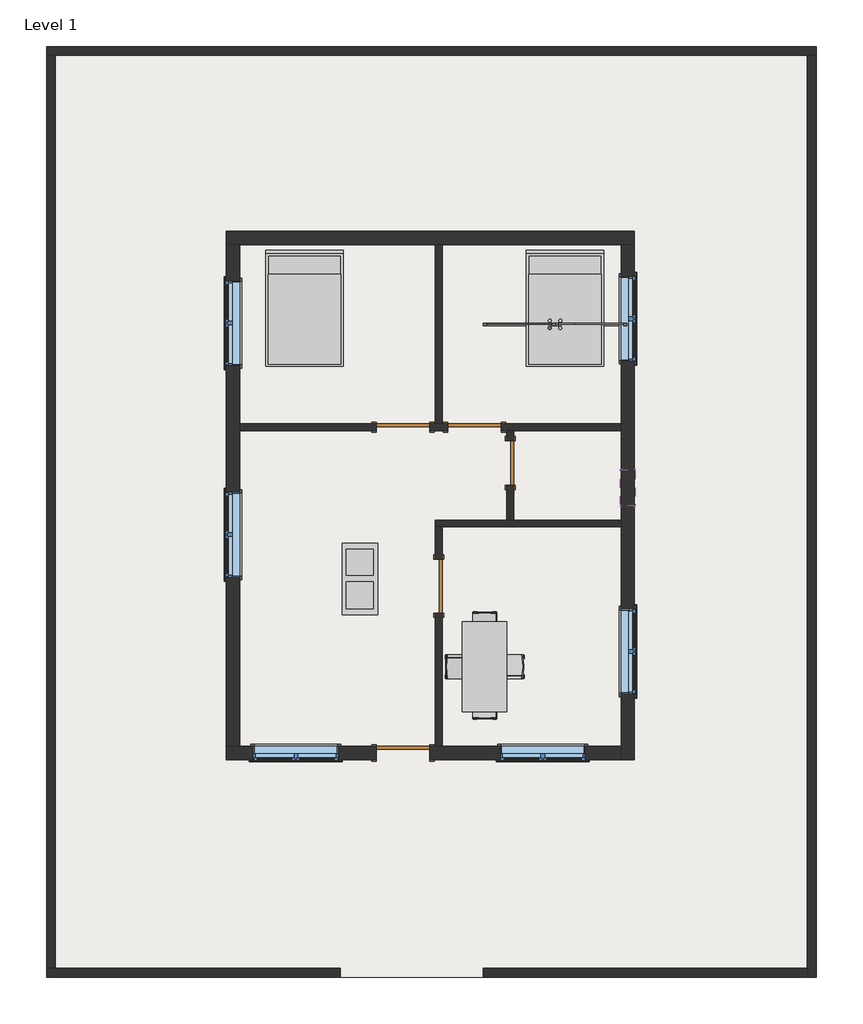
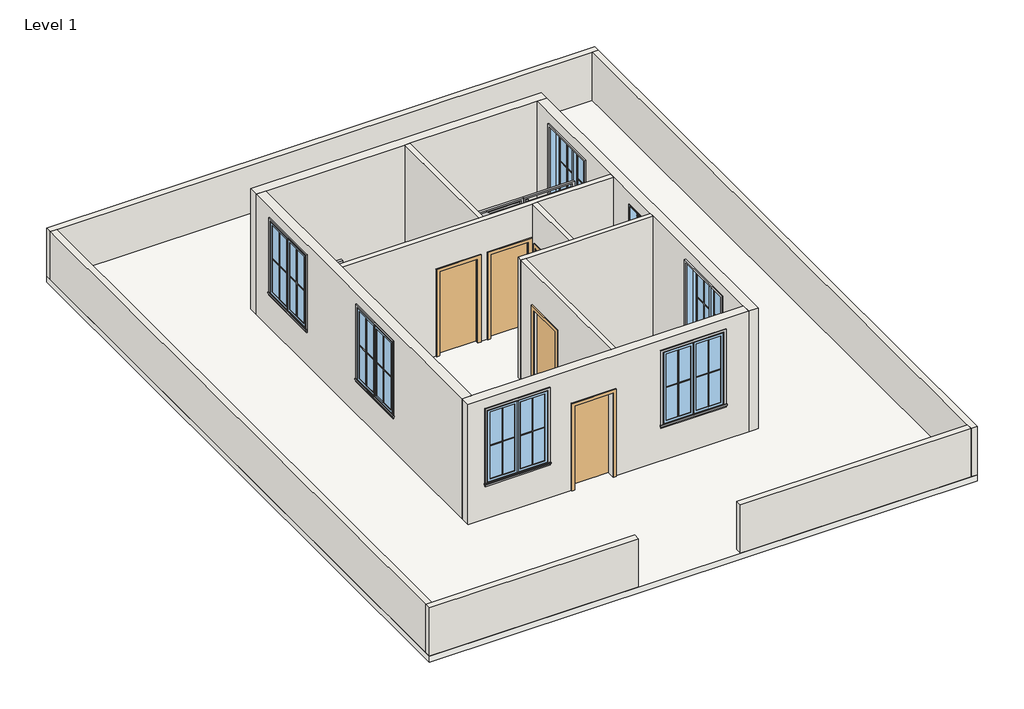
# One storey, incomplete: 26 proxies, 14 walls, 7 windows, 5 doors, 3 furniture elements, 1 slab.
"""IFC4 building model written with IfcOpenShell, lengths in millimetres."""

from ifc_helpers import new_model, si_unit, frame, origin, origin_with_axes, place, context, project, spatial, polyline, outline, extrude, faceted_brep, transform, mapped, element, save
from components import generic_models_113f6068, muntin_pattern_2x2_muntin_pattern_2x2_bff912c5, muntin_pattern_2x2_muntin_pattern_2x2_c2194282, trim_window_exterior_flat_with_sill_e04b3088, trim_window_interior_flat_picture_frame_2a7685fe, coffee_table_with_brass_mullions_11320_coffee_table_with_5962bef7, door_305aa2a5, door_e5f9f3c4, door_0ca8825f, door_f2b275c1, bed_17739_bed_17739_15c61121, dining_table_w_chairs_11374_0cdfc61b, window_9ac97e1a, window_f2d8fef0

model = new_model("IFC4")

# Units and contexts
model_context = context("Model", 3, world=origin())
ifc_project = project(units=[si_unit("LENGTHUNIT", "METRE", prefix="MILLI")], contexts=[model_context])

# Site, building, storey
site = spatial("IfcSite", under=ifc_project)
building = spatial("IfcBuilding", under=site)
storey = spatial("IfcBuildingStorey", under=building, Name="Level 1", Elevation=0.0)

# Proxies
placement = place(None, origin())
generic_models_shape = generic_models_113f6068(model_context)
element("IfcBuildingElementProxy", 1, Name="Generic Models", at=placement, inside=storey, context=model_context, shape_type="MappedRepresentation", body=[
    mapped(generic_models_shape, transform((866.6812648, 2380.4936265, 0.0), x_axis=(1.0, 0.0, 0.0), y_axis=(0.0, 1.0, 0.0), z_axis=(0.0, 0.0, 1.0))),
])
muntin_pattern_2x2_muntin_pattern_2x2_shape = muntin_pattern_2x2_muntin_pattern_2x2_bff912c5(model_context)
element("IfcBuildingElementProxy", 2, Name="Muntin Pattern_2x2 : Muntin Pattern_2x2", ObjectType="Muntin Pattern_2x2 : Muntin Pattern_2x2", at=placement, inside=storey, context=model_context, shape_type="MappedRepresentation", body=[
    mapped(muntin_pattern_2x2_muntin_pattern_2x2_shape, transform((-4718.1437352, -1580.3188735, 984.25), x_axis=(0.0, 1.0, 0.0), y_axis=(-1.0, 0.0, 0.0), z_axis=(0.0, 0.0, 1.0))),
])
element("IfcBuildingElementProxy", 3, Name="Muntin Pattern_2x2 : Muntin Pattern_2x2", ObjectType="Muntin Pattern_2x2 : Muntin Pattern_2x2", at=placement, inside=storey, context=model_context, shape_type="MappedRepresentation", body=[
    mapped(muntin_pattern_2x2_muntin_pattern_2x2_shape, transform((-3186.2062352, -5039.4813735, 984.25), x_axis=(-1.0, 0.0, 0.0), y_axis=(0.0, -1.0, 0.0), z_axis=(0.0, 0.0, 1.0))),
])
element("IfcBuildingElementProxy", 4, Name="Muntin Pattern_2x2 : Muntin Pattern_2x2", ObjectType="Muntin Pattern_2x2 : Muntin Pattern_2x2", at=placement, inside=storey, context=model_context, shape_type="MappedRepresentation", body=[
    mapped(muntin_pattern_2x2_muntin_pattern_2x2_shape, transform((1017.4937648, -5039.4813735, 984.25), x_axis=(-1.0, 0.0, 0.0), y_axis=(0.0, -1.0, 0.0), z_axis=(0.0, 0.0, 1.0))),
])
element("IfcBuildingElementProxy", 5, Name="Muntin Pattern_2x2 : Muntin Pattern_2x2", ObjectType="Muntin Pattern_2x2 : Muntin Pattern_2x2", at=placement, inside=storey, context=model_context, shape_type="MappedRepresentation", body=[
    mapped(muntin_pattern_2x2_muntin_pattern_2x2_shape, transform((2209.7062648, -2847.1438735, 984.25), x_axis=(0.0, -1.0, 0.0), y_axis=(1.0, 0.0, 0.0), z_axis=(0.0, 0.0, 1.0))),
])
element("IfcBuildingElementProxy", 6, Name="Muntin Pattern_2x2 : Muntin Pattern_2x2", ObjectType="Muntin Pattern_2x2 : Muntin Pattern_2x2", at=placement, inside=storey, context=model_context, shape_type="MappedRepresentation", body=[
    mapped(muntin_pattern_2x2_muntin_pattern_2x2_shape, transform((2209.7062648, 2817.0561265, 984.25), x_axis=(0.0, -1.0, 0.0), y_axis=(1.0, 0.0, 0.0), z_axis=(0.0, 0.0, 1.0))),
])
element("IfcBuildingElementProxy", 7, Name="Muntin Pattern_2x2 : Muntin Pattern_2x2", ObjectType="Muntin Pattern_2x2 : Muntin Pattern_2x2", at=placement, inside=storey, context=model_context, shape_type="MappedRepresentation", body=[
    mapped(muntin_pattern_2x2_muntin_pattern_2x2_shape, transform((-4718.1437352, 2020.1311265, 984.25), x_axis=(0.0, 1.0, 0.0), y_axis=(-1.0, 0.0, 0.0), z_axis=(0.0, 0.0, 1.0))),
])
muntin_pattern_2x2_muntin_pattern_2x2_2_shape = muntin_pattern_2x2_muntin_pattern_2x2_c2194282(model_context)
element("IfcBuildingElementProxy", 8, Name="Muntin Pattern_2x2 : Muntin Pattern_2x2", ObjectType="Muntin Pattern_2x2 : Muntin Pattern_2x2", at=placement, inside=storey, context=model_context, shape_type="MappedRepresentation", body=[
    mapped(muntin_pattern_2x2_muntin_pattern_2x2_2_shape, transform((-4718.1437352, -859.5938735, 984.25), x_axis=(0.0, -1.0, 0.0), y_axis=(1.0, 0.0, 0.0), z_axis=(0.0, 0.0, 1.0))),
])
element("IfcBuildingElementProxy", 9, Name="Muntin Pattern_2x2 : Muntin Pattern_2x2", ObjectType="Muntin Pattern_2x2 : Muntin Pattern_2x2", at=placement, inside=storey, context=model_context, shape_type="MappedRepresentation", body=[
    mapped(muntin_pattern_2x2_muntin_pattern_2x2_2_shape, transform((-3906.9312352, -5039.4813735, 984.25), x_axis=(1.0, 0.0, 0.0), y_axis=(0.0, 1.0, 0.0), z_axis=(0.0, 0.0, 1.0))),
])
element("IfcBuildingElementProxy", 10, Name="Muntin Pattern_2x2 : Muntin Pattern_2x2", ObjectType="Muntin Pattern_2x2 : Muntin Pattern_2x2", at=placement, inside=storey, context=model_context, shape_type="MappedRepresentation", body=[
    mapped(muntin_pattern_2x2_muntin_pattern_2x2_2_shape, transform((296.7687648, -5039.4813735, 984.25), x_axis=(1.0, 0.0, 0.0), y_axis=(0.0, 1.0, 0.0), z_axis=(0.0, 0.0, 1.0))),
])
element("IfcBuildingElementProxy", 11, Name="Muntin Pattern_2x2 : Muntin Pattern_2x2", ObjectType="Muntin Pattern_2x2 : Muntin Pattern_2x2", at=placement, inside=storey, context=model_context, shape_type="MappedRepresentation", body=[
    mapped(muntin_pattern_2x2_muntin_pattern_2x2_2_shape, transform((2209.7062648, -3567.8688735, 984.25), x_axis=(0.0, 1.0, 0.0), y_axis=(-1.0, 0.0, 0.0), z_axis=(0.0, 0.0, 1.0))),
])
element("IfcBuildingElementProxy", 12, Name="Muntin Pattern_2x2 : Muntin Pattern_2x2", ObjectType="Muntin Pattern_2x2 : Muntin Pattern_2x2", at=placement, inside=storey, context=model_context, shape_type="MappedRepresentation", body=[
    mapped(muntin_pattern_2x2_muntin_pattern_2x2_2_shape, transform((2209.7062648, 2096.3311265, 984.25), x_axis=(0.0, 1.0, 0.0), y_axis=(-1.0, 0.0, 0.0), z_axis=(0.0, 0.0, 1.0))),
])
element("IfcBuildingElementProxy", 13, Name="Muntin Pattern_2x2 : Muntin Pattern_2x2", ObjectType="Muntin Pattern_2x2 : Muntin Pattern_2x2", at=placement, inside=storey, context=model_context, shape_type="MappedRepresentation", body=[
    mapped(muntin_pattern_2x2_muntin_pattern_2x2_2_shape, transform((-4718.1437352, 2740.8561265, 984.25), x_axis=(0.0, -1.0, 0.0), y_axis=(1.0, 0.0, 0.0), z_axis=(0.0, 0.0, 1.0))),
])
trim_window_exterior_flat_with_sill_shape = trim_window_exterior_flat_with_sill_e04b3088(model_context)
element("IfcBuildingElementProxy", 14, Name="Trim-Window-Exterior-Flat : with Sill", ObjectType="Trim-Window-Exterior-Flat : with Sill", at=placement, inside=storey, context=model_context, shape_type="MappedRepresentation", body=[
    mapped(trim_window_exterior_flat_with_sill_shape, transform((-4727.6687352, -1219.9563735, 2743.2), x_axis=(0.0, -1.0, 0.0), y_axis=(0.0, 0.0, 1.0), z_axis=(-1.0, 0.0, 0.0))),
])
element("IfcBuildingElementProxy", 15, Name="Trim-Window-Exterior-Flat : with Sill", ObjectType="Trim-Window-Exterior-Flat : with Sill", at=placement, inside=storey, context=model_context, shape_type="MappedRepresentation", body=[
    mapped(trim_window_exterior_flat_with_sill_shape, transform((-3546.5687352, -5049.0063735, 2743.2), x_axis=(1.0, 0.0, 0.0), y_axis=(0.0, 0.0, 1.0), z_axis=(0.0, -1.0, 0.0))),
])
element("IfcBuildingElementProxy", 16, Name="Trim-Window-Exterior-Flat : with Sill", ObjectType="Trim-Window-Exterior-Flat : with Sill", at=placement, inside=storey, context=model_context, shape_type="MappedRepresentation", body=[
    mapped(trim_window_exterior_flat_with_sill_shape, transform((657.1312648, -5049.0063735, 2743.2), x_axis=(1.0, 0.0, 0.0), y_axis=(0.0, 0.0, 1.0), z_axis=(0.0, -1.0, 0.0))),
])
element("IfcBuildingElementProxy", 17, Name="Trim-Window-Exterior-Flat : with Sill", ObjectType="Trim-Window-Exterior-Flat : with Sill", at=placement, inside=storey, context=model_context, shape_type="MappedRepresentation", body=[
    mapped(trim_window_exterior_flat_with_sill_shape, transform((2219.2312648, -3207.5063735, 2743.2), x_axis=(0.0, 1.0, 0.0), y_axis=(0.0, 0.0, 1.0), z_axis=(1.0, 0.0, 0.0))),
])
element("IfcBuildingElementProxy", 18, Name="Trim-Window-Exterior-Flat : with Sill", ObjectType="Trim-Window-Exterior-Flat : with Sill", at=placement, inside=storey, context=model_context, shape_type="MappedRepresentation", body=[
    mapped(trim_window_exterior_flat_with_sill_shape, transform((2219.2312648, 2456.6936265, 2743.2), x_axis=(0.0, 1.0, 0.0), y_axis=(0.0, 0.0, 1.0), z_axis=(1.0, 0.0, 0.0))),
])
element("IfcBuildingElementProxy", 19, Name="Trim-Window-Exterior-Flat : with Sill", ObjectType="Trim-Window-Exterior-Flat : with Sill", at=placement, inside=storey, context=model_context, shape_type="MappedRepresentation", body=[
    mapped(trim_window_exterior_flat_with_sill_shape, transform((-4727.6687352, 2380.4936265, 2743.2), x_axis=(0.0, -1.0, 0.0), y_axis=(0.0, 0.0, 1.0), z_axis=(-1.0, 0.0, 0.0))),
])
trim_window_interior_flat_picture_frame_shape = trim_window_interior_flat_picture_frame_2a7685fe(model_context)
element("IfcBuildingElementProxy", 20, Name="Trim-Window-Interior-Flat : Picture Frame", ObjectType="Trim-Window-Interior-Flat : Picture Frame", at=placement, inside=storey, context=model_context, shape_type="MappedRepresentation", body=[
    mapped(trim_window_interior_flat_picture_frame_shape, transform((-4499.0687352, -1219.9563735, 2743.2), x_axis=(0.0, 1.0, 0.0), y_axis=(0.0, 0.0, 1.0), z_axis=(1.0, 0.0, 0.0))),
])
element("IfcBuildingElementProxy", 21, Name="Trim-Window-Interior-Flat : Picture Frame", ObjectType="Trim-Window-Interior-Flat : Picture Frame", at=placement, inside=storey, context=model_context, shape_type="MappedRepresentation", body=[
    mapped(trim_window_interior_flat_picture_frame_shape, transform((-3546.5687352, -4820.4063735, 2743.2), x_axis=(-1.0, 0.0, 0.0), y_axis=(0.0, 0.0, 1.0), z_axis=(0.0, 1.0, 0.0))),
])
element("IfcBuildingElementProxy", 22, Name="Trim-Window-Interior-Flat : Picture Frame", ObjectType="Trim-Window-Interior-Flat : Picture Frame", at=placement, inside=storey, context=model_context, shape_type="MappedRepresentation", body=[
    mapped(trim_window_interior_flat_picture_frame_shape, transform((657.1312648, -4820.4063735, 2743.2), x_axis=(-1.0, 0.0, 0.0), y_axis=(0.0, 0.0, 1.0), z_axis=(0.0, 1.0, 0.0))),
])
element("IfcBuildingElementProxy", 23, Name="Trim-Window-Interior-Flat : Picture Frame", ObjectType="Trim-Window-Interior-Flat : Picture Frame", at=placement, inside=storey, context=model_context, shape_type="MappedRepresentation", body=[
    mapped(trim_window_interior_flat_picture_frame_shape, transform((1990.6312648, -3207.5063735, 2743.2), x_axis=(0.0, -1.0, 0.0), y_axis=(0.0, 0.0, 1.0), z_axis=(-1.0, 0.0, 0.0))),
])
element("IfcBuildingElementProxy", 24, Name="Trim-Window-Interior-Flat : Picture Frame", ObjectType="Trim-Window-Interior-Flat : Picture Frame", at=placement, inside=storey, context=model_context, shape_type="MappedRepresentation", body=[
    mapped(trim_window_interior_flat_picture_frame_shape, transform((1990.6312648, 2456.6936265, 2743.2), x_axis=(0.0, -1.0, 0.0), y_axis=(0.0, 0.0, 1.0), z_axis=(-1.0, 0.0, 0.0))),
])
element("IfcBuildingElementProxy", 25, Name="Trim-Window-Interior-Flat : Picture Frame", ObjectType="Trim-Window-Interior-Flat : Picture Frame", at=placement, inside=storey, context=model_context, shape_type="MappedRepresentation", body=[
    mapped(trim_window_interior_flat_picture_frame_shape, transform((-4499.0687352, 2380.4936265, 2743.2), x_axis=(0.0, 1.0, 0.0), y_axis=(0.0, 0.0, 1.0), z_axis=(1.0, 0.0, 0.0))),
])
coffee_table_with_brass_mullions_11320_coffee_table_with_shape = coffee_table_with_brass_mullions_11320_coffee_table_with_5962bef7(model_context)
element("IfcBuildingElementProxy", 26, Name="coffee_table_with_brass_mullions_11320 : coffee_table_with_brass_mullions_11320", ObjectType="coffee_table_with_brass_mullions_11320 : coffee_table_with_brass_mullions_11320", at=placement, inside=storey, context=model_context, shape_type="MappedRepresentation", body=[
    mapped(coffee_table_with_brass_mullions_11320_coffee_table_with_shape, transform((-2022.5687352, -1334.2563735, 0.0), x_axis=(0.0, 1.0, 0.0), y_axis=(-1.0, 0.0, 0.0), z_axis=(0.0, 0.0, 1.0))),
])

# Doors
door_shape = door_305aa2a5(model_context)
element("IfcDoor", 27, ObjectType="Single-Flush : 36\" x 84\"", at=placement, inside=storey, context=model_context, shape_type="MappedRepresentation", body=[
    mapped(door_shape, transform((-1114.5187352, -2096.2563735, 0.0), x_axis=(0.0, 1.0, 0.0), y_axis=(-1.0, 0.0, 0.0), z_axis=(0.0, 0.0, 1.0))),
])
element("IfcDoor", 28, ObjectType="Single-Flush : 36\" x 84\"", at=placement, inside=storey, context=model_context, shape_type="MappedRepresentation", body=[
    mapped(door_shape, transform((-1724.1187352, 608.8436265, 0.0), x_axis=(-1.0, 0.0, 0.0), y_axis=(0.0, -1.0, 0.0), z_axis=(0.0, 0.0, 1.0))),
])
door_2_shape = door_e5f9f3c4(model_context)
element("IfcDoor", 29, ObjectType="Single-Flush : 36\" x 84\"", at=placement, inside=storey, context=model_context, shape_type="MappedRepresentation", body=[
    mapped(door_2_shape, transform((-504.9187352, 608.8436265, 0.0), x_axis=(1.0, 0.0, 0.0), y_axis=(0.0, 1.0, 0.0), z_axis=(0.0, 0.0, 1.0))),
])
door_3_shape = door_0ca8825f(model_context)
element("IfcDoor", 30, ObjectType="Single-Flush : 36\" x 84\"", at=placement, inside=storey, context=model_context, shape_type="MappedRepresentation", body=[
    mapped(door_3_shape, transform((-1724.1187352, -4934.7063735, 0.0), x_axis=(1.0, 0.0, 0.0), y_axis=(0.0, 1.0, 0.0), z_axis=(0.0, 0.0, 1.0))),
])
door_4_shape = door_f2b275c1(model_context)
element("IfcDoor", 31, ObjectType="Single-Flush : DOOR 2'6\"", at=placement, inside=storey, context=model_context, shape_type="MappedRepresentation", body=[
    mapped(door_4_shape, transform((104.6812648, -0.7563735, 0.0), x_axis=(0.0, 1.0, 0.0), y_axis=(-1.0, 0.0, 0.0), z_axis=(0.0, 0.0, 1.0))),
])

# Furniture
bed_17739_bed_17739_shape = bed_17739_bed_17739_15c61121(model_context)
element("IfcFurniture", 32, ObjectType="Bed_17739 : Bed_17739", at=placement, inside=storey, context=model_context, shape_type="MappedRepresentation", body=[
    mapped(bed_17739_bed_17739_shape, transform((-3400.5187352, 2609.0936265, 0.0), x_axis=(1.0, 0.0, 0.0), y_axis=(0.0, 1.0, 0.0), z_axis=(0.0, 0.0, 1.0))),
])
element("IfcFurniture", 33, ObjectType="Bed_17739 : Bed_17739", at=placement, inside=storey, context=model_context, shape_type="MappedRepresentation", body=[
    mapped(bed_17739_bed_17739_shape, transform((1038.1312648, 2609.0936265, 0.0), x_axis=(1.0, 0.0, 0.0), y_axis=(0.0, 1.0, 0.0), z_axis=(0.0, 0.0, 1.0))),
])
dining_table_w_chairs_11374_shape = dining_table_w_chairs_11374_0cdfc61b(model_context)
element("IfcFurniture", 34, ObjectType="Dining_Table_w_Chairs_11374", at=placement, inside=storey, context=model_context, shape_type="MappedRepresentation", body=[
    mapped(dining_table_w_chairs_11374_shape, transform((-238.2576574, -3486.1221401, 0.0), x_axis=(0.0, 1.0, 0.0), y_axis=(-1.0, 0.0, 0.0), z_axis=(0.0, 0.0, 1.0))),
])

# Slab
element("IfcSlab", 35, ObjectType="FLOOR 6\"", at=placement, inside=storey, context=model_context, shape_type="SweptSolid", body=[
    extrude(outline(polyline([(5315.4099973, 7091.2559969), (5315.4099973, -8758.3440031), (-7790.9900027, -8758.3440031), (-7790.9900027, 7091.2559969), (5315.4099973, 7091.2559969)])), frame((0.0, 0.0, -152.4), z_axis=(0.0, 0.0, 1.0), x_axis=(1.0, 0.0, 0.0)), (0.0, 0.0, 1.0), 152.4),
])

# Walls
element("IfcWall", 36, ObjectType="CMD 6\"", at=placement, inside=storey, context=model_context, shape_type="Brep", body=[
    faceted_brep([(-7790.9900027, 6938.8559969, 0.0), (-7638.5900027, 6938.8559969, 0.0), (5163.0099973, 6938.8559969, 0.0), (5315.4099973, 6938.8559969, 0.0), (5315.4099973, 6938.8559969, 1219.2), (5163.0099973, 6938.8559969, 1219.2), (-7638.5900027, 6938.8559969, 1219.2), (-7790.9900027, 6938.8559969, 1219.2), (-7790.9900027, 7091.2559969, 0.0), (-7790.9900027, 7091.2559969, 1219.2), (5315.4099973, 7091.2559969, 1219.2), (5315.4099973, 7091.2559969, 0.0)], [[[0, 1, 2, 3, 4, 5, 6, 7]], [[8, 9, 10, 11]], [[3, 2, 1, 0, 8, 11]], [[7, 6, 5, 4, 10, 9]], [[4, 3, 11, 10]], [[0, 7, 9, 8]]]),
])
element("IfcWall", 37, ObjectType="CMD 6\"", at=placement, inside=storey, context=model_context, shape_type="Brep", body=[
    faceted_brep([(5163.0099973, 6938.8559969, 0.0), (5163.0099973, -8605.9440031, 0.0), (5163.0099973, -8758.3440031, 0.0), (5163.0099973, -8758.3440031, 1219.2), (5163.0099973, -8605.9440031, 1219.2), (5163.0099973, 6938.8559969, 1219.2), (5315.4099973, 6938.8559969, 0.0), (5315.4099973, 6938.8559969, 1219.2), (5315.4099973, -8758.3440031, 1219.2), (5315.4099973, -8758.3440031, 0.0)], [[[0, 1, 2, 3, 4, 5]], [[6, 7, 8, 9]], [[2, 1, 0, 6, 9]], [[5, 4, 3, 8, 7]], [[0, 5, 7, 6]], [[3, 2, 9, 8]]]),
])
element("IfcWall", 38, ObjectType="CMD 6\"", at=placement, inside=storey, context=model_context, shape_type="SweptSolid", body=[
    extrude(outline(polyline([(-352.5187352, -8605.9440031), (5163.0099973, -8605.9440031), (5163.0099973, -8758.3440031), (-352.5187352, -8758.3440031), (-352.5187352, -8605.9440031)])), origin_with_axes(), (0.0, 0.0, 1.0), 1219.2),
])
element("IfcWall", 39, ObjectType="CMD 6\"", at=placement, inside=storey, context=model_context, shape_type="SweptSolid", body=[
    extrude(outline(polyline([(-7638.5900027, 6938.8559969), (-7638.5900027, -8605.9440031), (-7790.9900027, -8605.9440031), (-7790.9900027, 6938.8559969), (-7638.5900027, 6938.8559969)])), origin_with_axes(), (0.0, 0.0, 1.0), 1219.2),
])
element("IfcWall", 40, ObjectType="CMD 6\"", at=placement, inside=storey, context=model_context, shape_type="Brep", body=[
    faceted_brep([(-2790.9187352, -8605.9440031, 0.0), (-7638.5900027, -8605.9440031, 0.0), (-7790.9900027, -8605.9440031, 0.0), (-7790.9900027, -8605.9440031, 1219.2), (-7638.5900027, -8605.9440031, 1219.2), (-2790.9187352, -8605.9440031, 1219.2), (-2790.9187352, -8758.3440031, 0.0), (-2790.9187352, -8758.3440031, 1219.2), (-7790.9900027, -8758.3440031, 1219.2), (-7790.9900027, -8758.3440031, 0.0)], [[[0, 1, 2, 3, 4, 5]], [[6, 7, 8, 9]], [[2, 1, 0, 6, 9]], [[5, 4, 3, 8, 7]], [[0, 5, 7, 6]], [[3, 2, 9, 8]]]),
])
element("IfcWall", 41, ObjectType="WALL 4.5\"", at=placement, inside=storey, context=model_context, shape_type="Brep", body=[
    faceted_brep([(-4499.0687352, 551.6936265, 0.0), (-2181.3187352, 551.6936265, 0.0), (-2181.3187352, 551.6936265, 2133.6), (-1266.9187352, 551.6936265, 2133.6), (-1266.9187352, 551.6936265, 0.0), (-962.1187352, 551.6936265, 0.0), (-962.1187352, 551.6936265, 2133.6), (-47.7187352, 551.6936265, 2133.6), (-47.7187352, 551.6936265, 0.0), (47.5312648, 551.6936265, 0.0), (161.8312648, 551.6936265, 0.0), (1990.6312648, 551.6936265, 0.0), (1990.6312648, 551.6936265, 3048.0), (161.8312648, 551.6936265, 3048.0), (47.5312648, 551.6936265, 3048.0), (-4499.0687352, 551.6936265, 3048.0), (-2181.3187352, 665.9936265, 2133.6), (-2181.3187352, 665.9936265, 0.0), (-4499.0687352, 665.9936265, 0.0), (-4499.0687352, 665.9936265, 3048.0), (-1171.6687352, 665.9936265, 3048.0), (-1057.3687352, 665.9936265, 3048.0), (1990.6312648, 665.9936265, 3048.0), (1990.6312648, 665.9936265, 0.0), (-47.7187352, 665.9936265, 0.0), (-47.7187352, 665.9936265, 2133.6), (-962.1187352, 665.9936265, 2133.6), (-962.1187352, 665.9936265, 0.0), (-1057.3687352, 665.9936265, 0.0), (-1171.6687352, 665.9936265, 0.0), (-1266.9187352, 665.9936265, 0.0), (-1266.9187352, 665.9936265, 2133.6)], [[[0, 1, 2, 3, 4, 5, 6, 7, 8, 9, 10, 11, 12, 13, 14, 15]], [[16, 17, 18, 19, 20, 21, 22, 23, 24, 25, 26, 27, 28, 29, 30, 31]], [[11, 10, 9, 8, 24, 23]], [[18, 17, 1, 0]], [[30, 29, 28, 27, 5, 4]], [[12, 11, 23, 22]], [[0, 15, 19, 18]], [[25, 24, 8, 7]], [[26, 25, 7, 6]], [[27, 26, 6, 5]], [[2, 1, 17, 16]], [[3, 2, 16, 31]], [[4, 3, 31, 30]], [[15, 14, 13, 12, 22, 21, 20, 19]]]),
])
element("IfcWall", 42, ObjectType="WALL 4.5\"", at=placement, inside=storey, context=model_context, shape_type="SweptSolid", body=[
    extrude(outline(polyline([(-1057.3687352, 3713.9936265), (-1057.3687352, 665.9936265), (-1171.6687352, 665.9936265), (-1171.6687352, 3713.9936265), (-1057.3687352, 3713.9936265)])), origin_with_axes(), (0.0, 0.0, 1.0), 3048.0),
])
element("IfcWall", 43, ObjectType="WALL 4.5\"", at=placement, inside=storey, context=model_context, shape_type="Brep", body=[
    faceted_brep([(1990.6312648, -972.3063735, 0.0), (161.8312648, -972.3063735, 0.0), (47.5312648, -972.3063735, 0.0), (-1171.6687352, -972.3063735, 0.0), (-1171.6687352, -972.3063735, 3048.0), (47.5312648, -972.3063735, 3048.0), (161.8312648, -972.3063735, 3048.0), (1990.6312648, -972.3063735, 3048.0), (1990.6312648, -1086.6063735, 0.0), (1990.6312648, -1086.6063735, 3048.0), (-1057.3687352, -1086.6063735, 3048.0), (-1171.6687352, -1086.6063735, 3048.0), (-1171.6687352, -1086.6063735, 0.0), (-1057.3687352, -1086.6063735, 0.0)], [[[0, 1, 2, 3, 4, 5, 6, 7]], [[8, 9, 10, 11, 12, 13]], [[3, 2, 1, 0, 8, 13, 12]], [[0, 7, 9, 8]], [[4, 3, 12, 11]], [[7, 6, 5, 4, 11, 10, 9]]]),
])
element("IfcWall", 44, ObjectType="WALL 4.5\"", at=placement, inside=storey, context=model_context, shape_type="SweptSolid", body=[
    extrude(outline(polyline([(-1086.6063735, 0.0), (-1639.0563735, 0.0), (-1639.0563735, 2133.6), (-2553.4563735, 2133.6), (-2553.4563735, 0.0), (-4820.4063735, 0.0), (-4820.4063735, 3048.0), (-1086.6063735, 3048.0), (-1086.6063735, 0.0)])), frame((-1171.6687352, 0.0, 0.0), z_axis=(1.0, 0.0, 0.0), x_axis=(0.0, 1.0, 0.0)), (0.0, 0.0, 1.0), 114.3),
])
element("IfcWall", 45, ObjectType="WALL 4.5\"", at=placement, inside=storey, context=model_context, shape_type="SweptSolid", body=[
    extrude(outline(polyline([(551.6936265, 0.0), (380.2436265, 0.0), (380.2436265, 2032.0), (-381.7563735, 2032.0), (-381.7563735, 0.0), (-972.3063735, 0.0), (-972.3063735, 3048.0), (551.6936265, 3048.0), (551.6936265, 0.0)])), frame((47.5312648, 0.0, 0.0), z_axis=(1.0, 0.0, 0.0), x_axis=(0.0, 1.0, 0.0)), (0.0, 0.0, 1.0), 114.3),
])
element("IfcWall", 46, ObjectType="WALL 9\"", at=placement, inside=storey, context=model_context, shape_type="Brep", body=[
    faceted_brep([(-4727.6687352, 3713.9936265, 0.0), (-4499.0687352, 3713.9936265, 0.0), (-1171.6687352, 3713.9936265, 0.0), (-1057.3687352, 3713.9936265, 0.0), (1990.6312648, 3713.9936265, 0.0), (2219.2312648, 3713.9936265, 0.0), (2219.2312648, 3713.9936265, 3048.0), (1990.6312648, 3713.9936265, 3048.0), (-1057.3687352, 3713.9936265, 3048.0), (-1171.6687352, 3713.9936265, 3048.0), (-4499.0687352, 3713.9936265, 3048.0), (-4727.6687352, 3713.9936265, 3048.0), (-4727.6687352, 3942.5936265, 0.0), (-4727.6687352, 3942.5936265, 3048.0), (2219.2312648, 3942.5936265, 3048.0), (2219.2312648, 3942.5936265, 0.0)], [[[0, 1, 2, 3, 4, 5, 6, 7, 8, 9, 10, 11]], [[12, 13, 14, 15]], [[5, 4, 3, 2, 1, 0, 12, 15]], [[6, 5, 15, 14]], [[0, 11, 13, 12]], [[11, 10, 9, 8, 7, 6, 14, 13]]]),
])
element("IfcWall", 47, ObjectType="WALL 9\"", at=placement, inside=storey, context=model_context, shape_type="Brep", body=[
    faceted_brep([(1990.6312648, 3713.9936265, 0.0), (1990.6312648, 665.9936265, 0.0), (1990.6312648, 551.6936265, 0.0), (1990.6312648, -972.3063735, 0.0), (1990.6312648, -1086.6063735, 0.0), (1990.6312648, -4820.4063735, 0.0), (1990.6312648, -5049.0063735, 0.0), (1990.6312648, -5049.0063735, 3048.0), (1990.6312648, -4820.4063735, 3048.0), (1990.6312648, -1086.6063735, 3048.0), (1990.6312648, -972.3063735, 3048.0), (1990.6312648, 551.6936265, 3048.0), (1990.6312648, 665.9936265, 3048.0), (1990.6312648, 3713.9936265, 3048.0), (1990.6312648, -3931.4063735, 2743.2), (1990.6312648, -3931.4063735, 914.4), (1990.6312648, -2483.6063735, 914.4), (1990.6312648, -2483.6063735, 2743.2), (1990.6312648, 1732.7936265, 2743.2), (1990.6312648, 1732.7936265, 914.4), (1990.6312648, 3180.5936265, 914.4), (1990.6312648, 3180.5936265, 2743.2), (1990.6312648, -115.0563735, 2743.2), (1990.6312648, -724.6563735, 2743.2), (1990.6312648, -724.6563735, 2133.6), (1990.6312648, -115.0563735, 2133.6), (2219.2312648, 3713.9936265, 0.0), (2219.2312648, 3713.9936265, 3048.0), (2219.2312648, -5049.0063735, 3048.0), (2219.2312648, -5049.0063735, 0.0), (2219.2312648, -3931.4063735, 2743.2), (2219.2312648, -2483.6063735, 2743.2), (2219.2312648, -2483.6063735, 914.4), (2219.2312648, -3931.4063735, 914.4), (2219.2312648, 1732.7936265, 2743.2), (2219.2312648, 3180.5936265, 2743.2), (2219.2312648, 3180.5936265, 914.4), (2219.2312648, 1732.7936265, 914.4), (2219.2312648, -115.0563735, 2743.2), (2219.2312648, -115.0563735, 2133.6), (2219.2312648, -724.6563735, 2133.6), (2219.2312648, -724.6563735, 2743.2)], [[[0, 1, 2, 3, 4, 5, 6, 7, 8, 9, 10, 11, 12, 13], [14, 15, 16, 17], [18, 19, 20, 21], [22, 23, 24, 25]], [[26, 27, 28, 29], [30, 31, 32, 33], [34, 35, 36, 37], [38, 39, 40, 41]], [[6, 5, 4, 3, 2, 1, 0, 26, 29]], [[0, 13, 27, 26]], [[7, 6, 29, 28]], [[15, 14, 30, 33]], [[16, 15, 33, 32]], [[17, 16, 32, 31]], [[14, 17, 31, 30]], [[19, 18, 34, 37]], [[20, 19, 37, 36]], [[21, 20, 36, 35]], [[18, 21, 35, 34]], [[39, 38, 22, 25]], [[40, 39, 25, 24]], [[41, 40, 24, 23]], [[38, 41, 23, 22]], [[13, 12, 11, 10, 9, 8, 7, 28, 27]]]),
])
element("IfcWall", 48, ObjectType="WALL 9\"", at=placement, inside=storey, context=model_context, shape_type="Brep", body=[
    faceted_brep([(1990.6312648, -4820.4063735, 0.0), (-1057.3687352, -4820.4063735, 0.0), (-1171.6687352, -4820.4063735, 0.0), (-1266.9187352, -4820.4063735, 0.0), (-1266.9187352, -4820.4063735, 2133.6), (-2181.3187352, -4820.4063735, 2133.6), (-2181.3187352, -4820.4063735, 0.0), (-4499.0687352, -4820.4063735, 0.0), (-4727.6687352, -4820.4063735, 0.0), (-4727.6687352, -4820.4063735, 3048.0), (-4499.0687352, -4820.4063735, 3048.0), (-1171.6687352, -4820.4063735, 3048.0), (-1057.3687352, -4820.4063735, 3048.0), (1990.6312648, -4820.4063735, 3048.0), (-4270.4687352, -4820.4063735, 2743.2), (-4270.4687352, -4820.4063735, 914.4), (-2822.6687352, -4820.4063735, 914.4), (-2822.6687352, -4820.4063735, 2743.2), (-66.7687352, -4820.4063735, 2743.2), (-66.7687352, -4820.4063735, 914.4), (1381.0312648, -4820.4063735, 914.4), (1381.0312648, -4820.4063735, 2743.2), (-1266.9187352, -5049.0063735, 2133.6), (-1266.9187352, -5049.0063735, 0.0), (1990.6312648, -5049.0063735, 0.0), (1990.6312648, -5049.0063735, 3048.0), (-4727.6687352, -5049.0063735, 3048.0), (-4727.6687352, -5049.0063735, 0.0), (-2181.3187352, -5049.0063735, 0.0), (-2181.3187352, -5049.0063735, 2133.6), (-4270.4687352, -5049.0063735, 2743.2), (-2822.6687352, -5049.0063735, 2743.2), (-2822.6687352, -5049.0063735, 914.4), (-4270.4687352, -5049.0063735, 914.4), (-66.7687352, -5049.0063735, 2743.2), (1381.0312648, -5049.0063735, 2743.2), (1381.0312648, -5049.0063735, 914.4), (-66.7687352, -5049.0063735, 914.4)], [[[0, 1, 2, 3, 4, 5, 6, 7, 8, 9, 10, 11, 12, 13], [14, 15, 16, 17], [18, 19, 20, 21]], [[22, 23, 24, 25, 26, 27, 28, 29], [30, 31, 32, 33], [34, 35, 36, 37]], [[28, 27, 8, 7, 6]], [[24, 23, 3, 2, 1, 0]], [[0, 13, 25, 24]], [[9, 8, 27, 26]], [[15, 14, 30, 33]], [[16, 15, 33, 32]], [[17, 16, 32, 31]], [[14, 17, 31, 30]], [[19, 18, 34, 37]], [[20, 19, 37, 36]], [[21, 20, 36, 35]], [[18, 21, 35, 34]], [[4, 3, 23, 22]], [[5, 4, 22, 29]], [[6, 5, 29, 28]], [[13, 12, 11, 10, 9, 26, 25]]]),
])
element("IfcWall", 49, ObjectType="WALL 9\"", at=placement, inside=storey, context=model_context, shape_type="Brep", body=[
    faceted_brep([(-4499.0687352, -4820.4063735, 0.0), (-4499.0687352, 551.6936265, 0.0), (-4499.0687352, 665.9936265, 0.0), (-4499.0687352, 3713.9936265, 0.0), (-4499.0687352, 3713.9936265, 3048.0), (-4499.0687352, 665.9936265, 3048.0), (-4499.0687352, 551.6936265, 3048.0), (-4499.0687352, -4820.4063735, 3048.0), (-4499.0687352, -496.0563735, 2743.2), (-4499.0687352, -496.0563735, 914.4), (-4499.0687352, -1943.8563735, 914.4), (-4499.0687352, -1943.8563735, 2743.2), (-4499.0687352, 3104.3936265, 2743.2), (-4499.0687352, 3104.3936265, 914.4), (-4499.0687352, 1656.5936265, 914.4), (-4499.0687352, 1656.5936265, 2743.2), (-4727.6687352, -4820.4063735, 0.0), (-4727.6687352, -4820.4063735, 3048.0), (-4727.6687352, 3713.9936265, 3048.0), (-4727.6687352, 3713.9936265, 0.0), (-4727.6687352, -496.0563735, 2743.2), (-4727.6687352, -1943.8563735, 2743.2), (-4727.6687352, -1943.8563735, 914.4), (-4727.6687352, -496.0563735, 914.4), (-4727.6687352, 3104.3936265, 2743.2), (-4727.6687352, 1656.5936265, 2743.2), (-4727.6687352, 1656.5936265, 914.4), (-4727.6687352, 3104.3936265, 914.4)], [[[0, 1, 2, 3, 4, 5, 6, 7], [8, 9, 10, 11], [12, 13, 14, 15]], [[16, 17, 18, 19], [20, 21, 22, 23], [24, 25, 26, 27]], [[3, 2, 1, 0, 16, 19]], [[4, 3, 19, 18]], [[0, 7, 17, 16]], [[9, 8, 20, 23]], [[10, 9, 23, 22]], [[11, 10, 22, 21]], [[8, 11, 21, 20]], [[13, 12, 24, 27]], [[14, 13, 27, 26]], [[15, 14, 26, 25]], [[12, 15, 25, 24]], [[7, 6, 5, 4, 18, 17]]]),
])

# Windows
window_shape = window_9ac97e1a(model_context)
element("IfcWindow", 50, ObjectType="Window-Casement-Double : 57\" x 72\"", at=placement, inside=storey, context=model_context, shape_type="MappedRepresentation", body=[
    mapped(window_shape, transform((-4613.3687352, -1219.9563735, 0.0), x_axis=(0.0, 1.0, 0.0), y_axis=(-1.0, 0.0, 0.0), z_axis=(0.0, 0.0, 1.0))),
])
element("IfcWindow", 51, ObjectType="Window-Casement-Double : 57\" x 72\"", at=placement, inside=storey, context=model_context, shape_type="MappedRepresentation", body=[
    mapped(window_shape, transform((-3546.5687352, -4934.7063735, 0.0), x_axis=(-1.0, 0.0, 0.0), y_axis=(0.0, -1.0, 0.0), z_axis=(0.0, 0.0, 1.0))),
])
element("IfcWindow", 52, ObjectType="Window-Casement-Double : 57\" x 72\"", at=placement, inside=storey, context=model_context, shape_type="MappedRepresentation", body=[
    mapped(window_shape, transform((657.1312648, -4934.7063735, 0.0), x_axis=(-1.0, 0.0, 0.0), y_axis=(0.0, -1.0, 0.0), z_axis=(0.0, 0.0, 1.0))),
])
element("IfcWindow", 53, ObjectType="Window-Casement-Double : 57\" x 72\"", at=placement, inside=storey, context=model_context, shape_type="MappedRepresentation", body=[
    mapped(window_shape, transform((2104.9312648, -3207.5063735, 0.0), x_axis=(0.0, -1.0, 0.0), y_axis=(1.0, 0.0, 0.0), z_axis=(0.0, 0.0, 1.0))),
])
element("IfcWindow", 54, ObjectType="Window-Casement-Double : 57\" x 72\"", at=placement, inside=storey, context=model_context, shape_type="MappedRepresentation", body=[
    mapped(window_shape, transform((2104.9312648, 2456.6936265, 0.0), x_axis=(0.0, -1.0, 0.0), y_axis=(1.0, 0.0, 0.0), z_axis=(0.0, 0.0, 1.0))),
])
element("IfcWindow", 55, ObjectType="Window-Casement-Double : 57\" x 72\"", at=placement, inside=storey, context=model_context, shape_type="MappedRepresentation", body=[
    mapped(window_shape, transform((-4613.3687352, 2380.4936265, 0.0), x_axis=(0.0, 1.0, 0.0), y_axis=(-1.0, 0.0, 0.0), z_axis=(0.0, 0.0, 1.0))),
])
window_2_shape = window_f2d8fef0(model_context)
element("IfcWindow", 56, ObjectType="Window-Louvers : 24\" x 24\"", at=placement, inside=storey, context=model_context, shape_type="MappedRepresentation", body=[
    mapped(window_2_shape, transform((2111.2812648, -419.8563735, 1219.2), x_axis=(0.0, -1.0, 0.0), y_axis=(1.0, 0.0, 0.0), z_axis=(0.0, 0.0, 1.0))),
])

save(model, "model.ifc")

# Revit data of these elements
# Type
#   sheet = none
#   pipe = none
#   handal = none
#   faram = none
#   Default Elevation = 0
# Type "Muntin Pattern_2x2 : Muntin Pattern_2x2"
#   Width [instance default] = 4' - 0"
#   Thickness = 0' - 0 1/2"
#   Height [instance default] = 4' - 0"
#   Distance = 0' - 0 3/4"
#   Interior Material [instance default] = none
#   Exterior Material [instance default] = none
#   Default Elevation = 0
# Type "Trim-Window-Exterior-Flat : with Sill"
#   Trim Width = 0' - 2 1/4"
#   Trim Thickness_Picture Frame = 0' - 1 1/4"
#   Trim Thickness_with Sill = 0' - 0 3/4"
#   Sill Thickness = 0' - 1 1/4"
#   Opening Width [instance default] = 2' - 0"
#   Opening Height [instance default] = 3' - 0"
#   Default Elevation = 4' - 0"
#   Sill = yes
#   Picture Frame = no
#   Trim Material [instance default] = none
# Type "Trim-Window-Interior-Flat : Picture Frame"
#   Trim Thickness_Picture Frame = 0' - 1 1/4"
#   Trim Width = 0' - 2 1/4"
#   Trim Thickness_with Sill = 0' - 0 3/4"
#   Sill Thickness = 0' - 1 1/4"
#   Opening Width [instance default] = 2' - 0"
#   Opening Height [instance default] = 3' - 0"
#   Default Elevation = 4' - 0"
#   Sill = no
#   Picture Frame = yes
#   Trim Material [instance default] = none
# Type "coffee_table_with_brass_mullions_11320 : coffee_table_with_brass_mullions_11320"
#   Default Elevation = 0
# Type "Single-Flush : 36\" x 84\""
#   Type Mark = "1"
#   Construction Type Id = "MDOOR"
#   Assembly Code = "C1020"
#   Analytic Construction = "Metal"
#   Thickness = 0' - 2"
#   Heat Transfer Coefficient (U) = 0.651978 BTU/(h·ft²·°F)
#   Height = 7' - 0"
#   Trim Projection Ext = 0' - 1"
#   Trim Projection Int = 0' - 1"
#   Trim Width = 0' - 3"
#   Width = 3' - 0"
#   Define Thermal Properties by = 1
#   Define Thermal Properties by = 1
#   Door Material = Door - Panel
#   Frame Material = Door - Frame
#   Visual Light Transmittance = 0
#   Solar Heat Gain Coefficient = 0
#   Function = (empty or 0)
#   Wall Closure = (empty or 0)
# Type "Single-Flush : DOOR 2'6\""
#   Type Mark = "8"
#   Construction Type Id = "MDOOR"
#   Assembly Code = "C1020"
#   Analytic Construction = "Metal"
#   Thickness = 0' - 2"
#   Heat Transfer Coefficient (U) = 0.651978 BTU/(h·ft²·°F)
#   Height = 6' - 8"
#   Trim Projection Ext = 0' - 1"
#   Trim Projection Int = 0' - 1"
#   Trim Width = 0' - 3"
#   Width = 2' - 6"
#   Define Thermal Properties by = 1
#   Door Material = Door - Panel
#   Frame Material = Door - Frame
#   Visual Light Transmittance = 0
#   Solar Heat Gain Coefficient = 0
#   Function = (empty or 0)
#   Wall Closure = (empty or 0)
# Type "Bed_17739 : Bed_17739"
#   Default Elevation = 0
# Type "Dining_Table_w_Chairs_11374"
#   Default Elevation = 0
#   Assembly Code = ""
# Type "FLOOR 6\""
#   Assembly Code = "B1010"
#   Function = 0
#   Layers, outside or top first: 0' - 6" no material (function 1)
# Type "CMD 6\""
#   Assembly Code = "B2010"
#   Layers, outside or top first: 0' - 6" no material (function 1)
# Type "WALL 4.5\""
#   Assembly Code = "B2010"
#   Layers, outside or top first: 0' - 4 1/2" no material (function 1)
# Type "WALL 9\""
#   Assembly Code = "B2010"
#   Layers, outside or top first: 0' - 9" no material (function 1)
# Type "Window-Casement-Double : 57\" x 72\""
#   Type Mark = "17"
#   Fire Rating = "0.5h"
#   Assembly Code = "B2020100"
#   Analytic Construction = "Double glazing - domestic"
#   Frame Extension [instance default] = 0' - 0 1/4"
#   Window Inset [instance default] = 0' - 0"
#   Wall Thickness [instance default] = 0' - 6"
#   Interior Wall Closure [instance default] = 0' - 2 1/4"
#   Half Width = 2' - 4 1/2"
#   Visual Light Transmittance = 0.81
#   Thermal Resistance (R) = 1.8146 (h·ft²·°F)/BTU
#   Solar Heat Gain Coefficient = 0.76
#   Rough Width = 4' - 9 1/2"
#   Rough Height = 6' - 0 1/2"
#   Height = 6' - 0"
#   Heat Transfer Coefficient (U) = 0.5511 BTU/(h·ft²·°F)
#   Exterior Wall Closure [instance default] = 0' - 1 1/4"
#   Extension Jamb [instance default] = 0' - 2 1/4"
#   Default Sill Height = 3' - 0"
#   Width = 4' - 9"
#   Define Thermal Properties by = 0
#   Muntin Visibility = yes
#   Interior Trim Visibility [instance default] = yes
#   Exterior Trim Visibility [instance default] = yes
#   Extension Jamb Visibility [instance default] = yes
#   Interior Trim Material = Wood - Stained
#   Muntin Pattern = Muntin Pattern_2x2 : Muntin Pattern_2x2
#   Interior Trim = Trim-Window-Interior-Flat : Picture Frame
#   Interior Frame Material = Wood - Stained
#   Glass Panel Material = Glass
#   Exterior Trim Material = Clad - White
#   Exterior Trim = Trim-Window-Exterior-Flat : with Sill
#   Exterior Frame Material = Clad - White
#   Wall Closure = (empty or 0)
# Type "Window-Louvers : 24\" x 24\""
#   Type Mark = "18"
#   Construction Type Id = "GSP4R"
#   Assembly Code = "B20"
#   Analytic Construction = "1/8 in Pilkington single glazing"
#   Visual Light Transmittance = 0.9
#   Thermal Resistance (R) = 1.53941 (h·ft²·°F)/BTU
#   Solar Heat Gain Coefficient = 0.78
#   Max Height = 1' - 11.74264"
#   Height = 2' - 0"
#   Heat Transfer Coefficient (U) = 0.6496 BTU/(h·ft²·°F)
#   Blade Width [instance default] = 1' - 10 1/2"
#   Blade Vertical Thickness = 0' - 0.35355"
#   Blade Thickness = 0' - 0 1/4"
#   Blade Spacing = 0' - 1 1/2"
#   Blade Height = 0' - 1.85355"
#   Blade Depth = 0' - 3"
#   Blade Angle = 45.00°
#   Default Sill Height = 3' - 0"
#   Trim Projection_Exterior = 0' - 0 1/2"
#   Trim Projection_Interior = 0' - 0 1/2"
#   Trim Width_Exterior = 0' - 1 1/2"
#   Trim Width_Interior = 0' - 1 1/2"
#   Width = 2' - 0"
#   Max Blade Count = 12
#   Define Thermal Properties by = 1
#   Blade Count = 12
#   Frame Material = Birch
#   Louver Material = Birch
#   Trim Exterior Material = Birch
#   Trim Interior Material = Birch
#   Wall Closure = (empty or 0)
# Element 1 (IfcBuildingElementProxy)
#   Phase Created = New Construction
# Elements 2, 3, 4, 5, 6, 7, 8, 9, 10, 11, 12, 13 (IfcBuildingElementProxy, "Muntin Pattern_2x2 : Muntin Pattern_2x2")
#   Width = 1' - 11 1/8"
#   Height = 5' - 6 1/2"
#   Interior Material = Wood - Stained
#   Exterior Material = Clad - White
#   Phase Created = New Construction
#   Materials on its faces: "Clad - White", "Wood - Stained"
# Elements 14, 15, 16, 17, 18, 19 (IfcBuildingElementProxy, "Trim-Window-Exterior-Flat : with Sill")
#   Opening Width = 4' - 9"
#   Opening Height = 6' - 0"
#   Trim Material = Clad - White
#   Phase Created = New Construction
#   Materials on its faces: "Clad - White"
# Elements 20, 21, 22, 23, 24, 25 (IfcBuildingElementProxy, "Trim-Window-Interior-Flat : Picture Frame")
#   Opening Width = 4' - 9"
#   Opening Height = 6' - 0"
#   Trim Material = Wood - Stained
#   Phase Created = New Construction
#   Materials on its faces: "Wood - Stained"
# Element 26 (IfcBuildingElementProxy, "coffee_table_with_brass_mullions_11320 : coffee_table_with_brass_mullions_11320")
#   Phase Created = New Construction
#   Materials on its faces: "Default Wall", "TABLE", "Glass", "Default"
# Elements 27, 28, 29, 30 (IfcDoor, "Single-Flush : 36\" x 84\"")
#   Phase Created = New Construction
#   Materials on its faces: "Door - Frame", "Door - Panel"
# Element 31 (IfcDoor, "Single-Flush : DOOR 2'6\"")
#   Phase Created = New Construction
#   Materials on its faces: "Door - Frame", "Door - Panel"
# Elements 32, 33 (IfcFurniture, "Bed_17739 : Bed_17739")
#   Phase Created = New Construction
#   Materials on its faces: "legs", "sheets", "bed frame", "Blanket"
# Element 34 (IfcFurniture, "Dining_Table_w_Chairs_11374")
#   Phase Created = New Construction
# Element 35 (IfcSlab, "FLOOR 6\"")
#   Height Offset From Level = 0' - 0"
#   Phase Created = New Construction
#   Materials on its faces: "Copper", "Default Floor", "Wood - Stained"
# Elements 36, 37, 40 (IfcWall, "CMD 6\"")
#   Top Offset = 0' - 0"
#   Base Offset = 0' - 0"
#   Unconnected Height = 4' - 0"
#   wall height = 4' - 0"
#   Phase Created = New Construction
#   Base Constraint = Level 1
#   Materials on its faces: "Clad - White", "Default Wall", "Copper"
# Elements 38, 39 (IfcWall, "CMD 6\"")
#   Top Offset = 0' - 0"
#   Base Offset = 0' - 0"
#   Unconnected Height = 4' - 0"
#   wall height = 4' - 0"
#   Phase Created = New Construction
#   Base Constraint = Level 1
#   Materials on its faces: "Default Wall", "Clad - White", "Copper"
# Elements 41, 42, 43, 44, 45 (IfcWall, "WALL 4.5\"")
#   Top Offset = 0' - 0"
#   Base Offset = 0' - 0"
#   Unconnected Height = 10' - 0"
#   wall height = 10' - 0"
#   Phase Created = New Construction
#   Base Constraint = Level 1
#   Materials on its faces: "Default Wall"
# Elements 46, 47, 48, 49 (IfcWall, "WALL 9\"")
#   Top Offset = 0' - 0"
#   Base Offset = 0' - 0"
#   Unconnected Height = 10' - 0"
#   wall height = 10' - 0"
#   Phase Created = New Construction
#   Base Constraint = Level 1
#   Materials on its faces: "Default Wall", "Parking Stripe"
# Element 50 (IfcWindow, "Window-Casement-Double : 57\" x 72\"")
#   Mark = "1"
#   Window Inset = 0' - 0"
#   Interior Wall Closure = 0' - 2 1/4"
#   Frame Extension = 0' - 0 1/4"
#   Exterior Wall Closure = 0' - 1 1/4"
#   Interior Trim Visibility = yes
#   Exterior Trim Visibility = yes
#   Phase Created = New Construction
#   Materials on its faces: "Wood - Stained", "Glass", "Clad - White"
# Element 51 (IfcWindow, "Window-Casement-Double : 57\" x 72\"")
#   Mark = "2"
#   Window Inset = 0' - 0"
#   Interior Wall Closure = 0' - 2 1/4"
#   Frame Extension = 0' - 0 1/4"
#   Exterior Wall Closure = 0' - 1 1/4"
#   Interior Trim Visibility = yes
#   Exterior Trim Visibility = yes
#   Phase Created = New Construction
#   Materials on its faces: "Wood - Stained", "Glass", "Clad - White"
# Element 52 (IfcWindow, "Window-Casement-Double : 57\" x 72\"")
#   Mark = "3"
#   Window Inset = 0' - 0"
#   Interior Wall Closure = 0' - 2 1/4"
#   Frame Extension = 0' - 0 1/4"
#   Exterior Wall Closure = 0' - 1 1/4"
#   Interior Trim Visibility = yes
#   Exterior Trim Visibility = yes
#   Phase Created = New Construction
#   Materials on its faces: "Wood - Stained", "Glass", "Clad - White"
# Element 53 (IfcWindow, "Window-Casement-Double : 57\" x 72\"")
#   Mark = "4"
#   Window Inset = 0' - 0"
#   Interior Wall Closure = 0' - 2 1/4"
#   Frame Extension = 0' - 0 1/4"
#   Exterior Wall Closure = 0' - 1 1/4"
#   Interior Trim Visibility = yes
#   Exterior Trim Visibility = yes
#   Phase Created = New Construction
#   Materials on its faces: "Wood - Stained", "Glass", "Clad - White"
# Element 54 (IfcWindow, "Window-Casement-Double : 57\" x 72\"")
#   Mark = "5"
#   Window Inset = 0' - 0"
#   Interior Wall Closure = 0' - 2 1/4"
#   Frame Extension = 0' - 0 1/4"
#   Exterior Wall Closure = 0' - 1 1/4"
#   Interior Trim Visibility = yes
#   Exterior Trim Visibility = yes
#   Phase Created = New Construction
#   Materials on its faces: "Wood - Stained", "Glass", "Clad - White"
# Element 55 (IfcWindow, "Window-Casement-Double : 57\" x 72\"")
#   Mark = "6"
#   Window Inset = 0' - 0"
#   Interior Wall Closure = 0' - 2 1/4"
#   Frame Extension = 0' - 0 1/4"
#   Exterior Wall Closure = 0' - 1 1/4"
#   Interior Trim Visibility = yes
#   Exterior Trim Visibility = yes
#   Phase Created = New Construction
#   Materials on its faces: "Wood - Stained", "Glass", "Clad - White"
# Element 56 (IfcWindow, "Window-Louvers : 24\" x 24\"")
#   Mark = "7"
#   Blade Width = 1' - 10 1/2"
#   Phase Created = New Construction
#   Materials on its faces: "Birch"
# Materials
#   "Door - Panel": class "Wood", colour RGB 210 159 95, transparency 0, Cost = 0
#   "Door - Frame": colour RGB 118 70 51, transparency 0, Cost = 0
#   "Wood - Stained": class "Wood", colour RGB 224 178 126, transparency 0, Cost = 0
#   "Glass": class "Glass", colour RGB 0 128 192, transparency 0.75, Description = "Soda Lime Glass", Cost = 0
#   "Clad - White": class "Wood", colour RGB 242 242 238, transparency 0, Cost = 0
#   "Birch": class "Wood", colour RGB 224 178 126, transparency 0, Description = "Betula Alleghaniensis", Cost = 0
#   "Default Wall": colour RGB 128 128 128, transparency 0, Cost = 0
#   "TABLE": class "Generic", colour RGB 120 120 120, transparency 0, Cost = 0
#   "Default": colour RGB 127 127 127, transparency 0, Cost = 0
#   "legs": colour RGB 90 73 37, transparency 0, Cost = 0
#   "sheets": colour RGB 200 195 176, transparency 0, Cost = 0
#   "bed frame": colour RGB 90 73 37, transparency 0, Cost = 0
#   "Blanket": class "System", colour RGB 59 0 1, transparency 0, Cost = 0
#   "Copper": class "Metal", colour RGB 0 0 0, transparency 0, Description = "Copper, matte finish", Cost = 0
#   "Default Floor": colour RGB 128 128 128, transparency 0, Cost = 0
#   "Parking Stripe": class "Paint", colour RGB 250 250 91, transparency 0, Cost = 0
